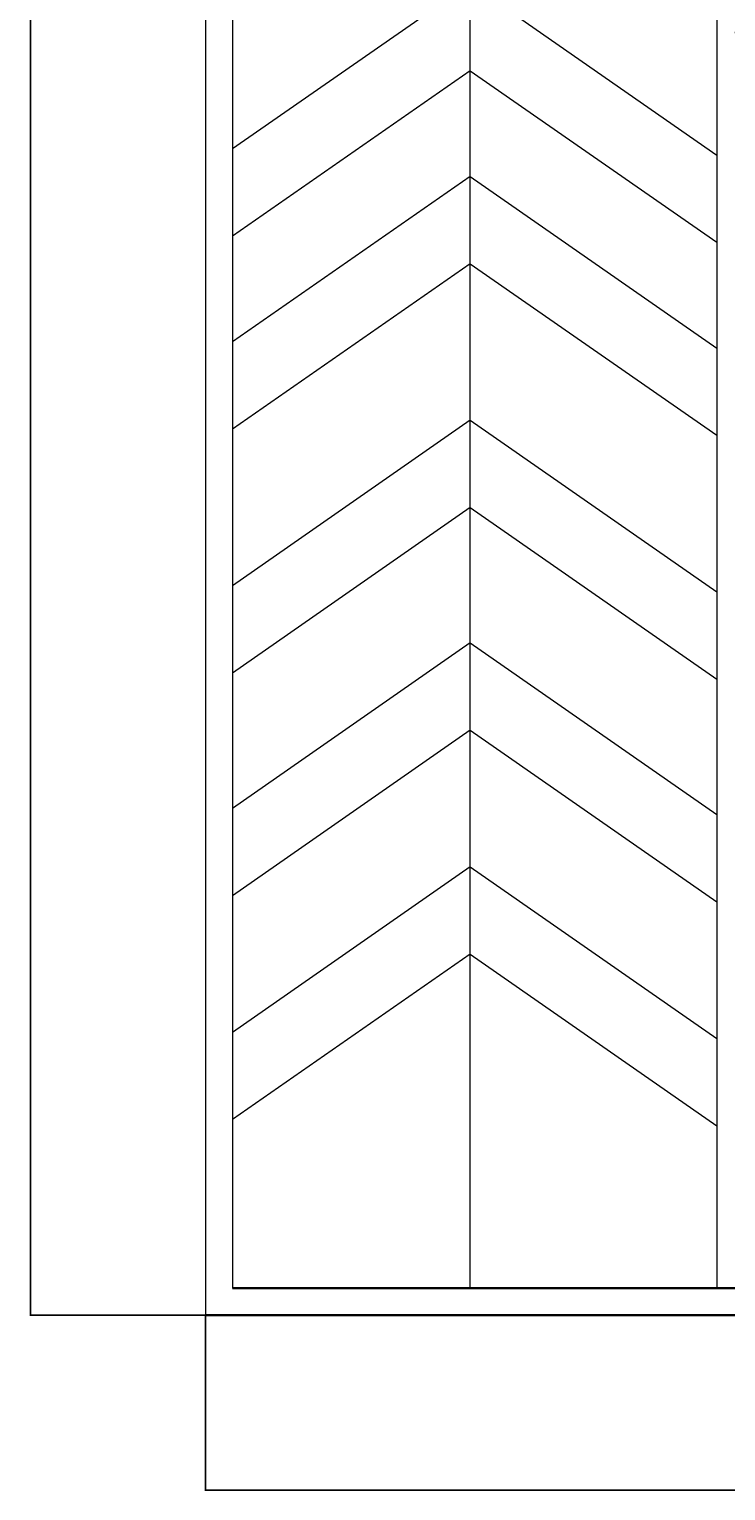
# Model space of a CAD drawing. Units: inches. Extents: x -46 to 1145, y -527 to 760.
# Tile 1 of 57: x -46 to 187, y -527 to -38. Entities that reach past the tile are written whole.
import ezdxf

# ---------------------------------------------------------------- set-up
doc = ezdxf.new("R2010")
doc.units = ezdxf.units.IN
doc.header["$MEASUREMENT"] = 0
for name, color, linetype, lineweight in [('A-ANNO-DIMS', 2, 'Continuous', 18), ('C-ROAD', 9, 'Continuous', 18), ('C-SITE', 7, 'Continuous', 30)]:
    doc.layers.add(name, color=color, linetype=linetype, lineweight=lineweight)
doc.styles.get("Standard").update_dxf_attribs({"font": 'arial.ttf'})
doc.dimstyles.get("Standard").update_dxf_attribs({"dimtxt": 0.18, "dimasz": 0.18, "dimexe": 0.18, "dimexo": 0.0625, "dimgap": 0.09, "dimtad": 0, "dimtih": 1, "dimtoh": 1, "dimdec": 0, "dimzin": 0, "dimdsep": 46, "dimlunit": 3, "dimtxsty": 'Standard', "dimcen": 0.09, "dimadec": 0, "dimazin": 0, "dimtfac": 1, "dimtdec": 0, "dimtofl": 0, "dimtmove": 0, "dimatfit": 3, "dimfxl": 1, "dimtolj": 1, "dimtzin": 0, "dimarcsym": 0})

# ---------------------------------------------------------------- blocks, each defined once
blk = doc.blocks.new('DRIVEWAY-CHEVRON')
for q in [(0, 2.03), (162, 0)]:
    blk.add_line((79.54, 57.38), q)
blk = doc.blocks.new('*D684')
at = {"layer": 'A-ANNO-DIMS', "color": 0, "lineweight": -2, "transparency": 16777216}
for p, q in [((12.56, -468.54), (12.56, -527.26)), ((1086.56, -468.54), (1086.56, -527.26)), ((12.74, -527.08), (549.21, -527.08)), ((1086.38, -527.08), (549.91, -527.08))]:
    blk.add_line(p, q, dxfattribs=at)
at = {"layer": 'A-ANNO-DIMS', "color": 0, "transparency": 16777216}
for points in [[(12.74, -527.05), (12.74, -527.11), (12.56, -527.08)], [(1086.38, -527.05), (1086.38, -527.11), (1086.56, -527.08)]]:
    blk.add_solid(points, dxfattribs=at)
at = {"layer": 'Defpoints', "color": 0, "transparency": 16777216}
for p in [(12.56, -468.48), (1086.56, -468.48), (1086.56, -527.08)]:
    blk.add_point(p, dxfattribs=at)
at = {"layer": 'A-ANNO-DIMS', "color": 0, "transparency": 16777216, "insert": (549.56, -527.08), "char_height": 0.18, "attachment_point": 5}
blk.add_mtext('\\A1;1074', dxfattribs=at)
blk = doc.blocks.new('*D685')
at = {"layer": 'A-ANNO-DIMS', "color": 0, "lineweight": -2, "transparency": 16777216}
for p, q in [((183.5, 700.89), (-46.22, 700.89)), ((-46.04, 700.71), (-46.04, 116.39)), ((-46.04, -468.3), (-46.04, 116.02)), ((12.5, -468.48), (-46.22, -468.48))]:
    blk.add_line(p, q, dxfattribs=at)
at = {"layer": 'A-ANNO-DIMS', "color": 0, "transparency": 16777216}
for points in [[(-46.07, 700.71), (-46.01, 700.71), (-46.04, 700.89)], [(-46.07, -468.3), (-46.01, -468.3), (-46.04, -468.48)]]:
    blk.add_solid(points, dxfattribs=at)
at = {"layer": 'Defpoints', "color": 0, "transparency": 16777216}
for p in [(-46.04, 700.89), (183.56, 700.89), (12.56, -468.48)]:
    blk.add_point(p, dxfattribs=at)
at = {"layer": 'A-ANNO-DIMS', "color": 0, "transparency": 16777216, "insert": (-46.04, 116.2), "char_height": 0.18, "attachment_point": 5}
blk.add_mtext('\\A1;1169.4', dxfattribs=at)
blk = doc.blocks.new('*D702')
at = {"layer": 'A-ANNO-DIMS', "color": 0, "lineweight": -2, "transparency": 16777216}
for p, q in [((189.63, -39.48), (1145.34, -39.48)), ((1145.16, -39.66), (1145.16, -249.3)), ((1145.16, -459.3), (1145.16, -249.66)), ((183.63, -459.48), (1145.34, -459.48))]:
    blk.add_line(p, q, dxfattribs=at)
at = {"layer": 'A-ANNO-DIMS', "color": 0, "transparency": 16777216}
for points in [[(1145.13, -39.66), (1145.19, -39.66), (1145.16, -39.48)], [(1145.13, -459.3), (1145.19, -459.3), (1145.16, -459.48)]]:
    blk.add_solid(points, dxfattribs=at)
at = {"layer": 'Defpoints', "color": 0, "transparency": 16777216}
for p in [(189.56, -39.48), (1145.16, -39.48), (183.56, -459.48)]:
    blk.add_point(p, dxfattribs=at)
at = {"layer": 'A-ANNO-DIMS', "color": 0, "transparency": 16777216, "insert": (1145.16, -249.48), "char_height": 0.18, "attachment_point": 5}
blk.add_mtext('\\A1;420', dxfattribs=at)

msp = doc.modelspace()

# ---------------------------------------------------------------- linework, layer by layer
at = {"layer": 'C-ROAD'}
for p, q in [((12.5637, 221.5176), (12.5637, -468.4824)), ((21.5637, 221.5176), (21.5637, -459.4824)), ((101.1042, -459.4824), (101.1042, 221.5176)), ((183.5637, 221.5176), (183.5637, -459.4824))]:
    msp.add_line(p, q, dxfattribs=at)
at = {"layer": 'C-SITE'}
for p, q in [((21.5637, -459.4824), (1077.5637, -459.4824)), ((12.5637, -468.4824), (1086.5637, -468.4824))]:
    msp.add_line(p, q, dxfattribs=at)

# ---------------------------------------------------------------- block references
at = {"layer": 'C-ROAD'}
for p in [(21.564, -80.4757), (21.564, -109.6688), (21.564, -145.0343), (21.564, -174.2274), (21.564, -226.575), (21.564, -255.768), (21.564, -301.0539), (21.564, -330.2469), (21.564, -375.9557), (21.564, -405.1488)]:
    msp.add_blockref('DRIVEWAY-CHEVRON', p, dxfattribs=at)

# ---------------------------------------------------------------- dimensions: what is measured, and where the dimension line sits
at = {"layer": 'A-ANNO-DIMS'}
for base, p1, p2, override, picture, middle in [((-46.0363, 700.8886), (12.5637, -468.4824), (183.5637, 700.8886), {"dimdec": 1, "dimlfac": 1, "dimrnd": 0, "dimzin": 0, "dimdsep": 46, "dimlunit": 2}, '*D685', (-46.0363, 116.2031)), ((1145.1637, -39.4824), (183.5637, -459.4824), (189.5637, -39.4824), {"dimdec": 0, "dimlfac": 1, "dimrnd": 0, "dimzin": 0, "dimdsep": 46, "dimlunit": 2}, '*D702', (1145.1637, -249.4824))]:
    dim = msp.add_linear_dim(base=base, p1=p1, p2=p2, angle=90, dimstyle='Standard', override=override, dxfattribs=at)
    dim.commit()
    dim.dimension.update_dxf_attribs({"geometry": picture, "text_midpoint": middle})
dim = msp.add_linear_dim(base=(1086.5637, -527.0824), p1=(12.5637, -468.4824), p2=(1086.5637, -468.4824), dimstyle='Standard', override={"dimdec": 0, "dimlfac": 1, "dimrnd": 0, "dimzin": 0, "dimdsep": 46, "dimlunit": 2}, dxfattribs=at)
dim.commit()
dim.dimension.update_dxf_attribs({"geometry": '*D684', "text_midpoint": (549.5637, -527.0824)})

doc.saveas('drawing.dxf')
